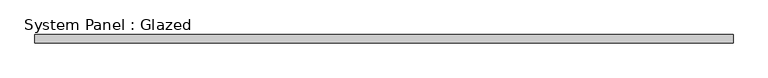
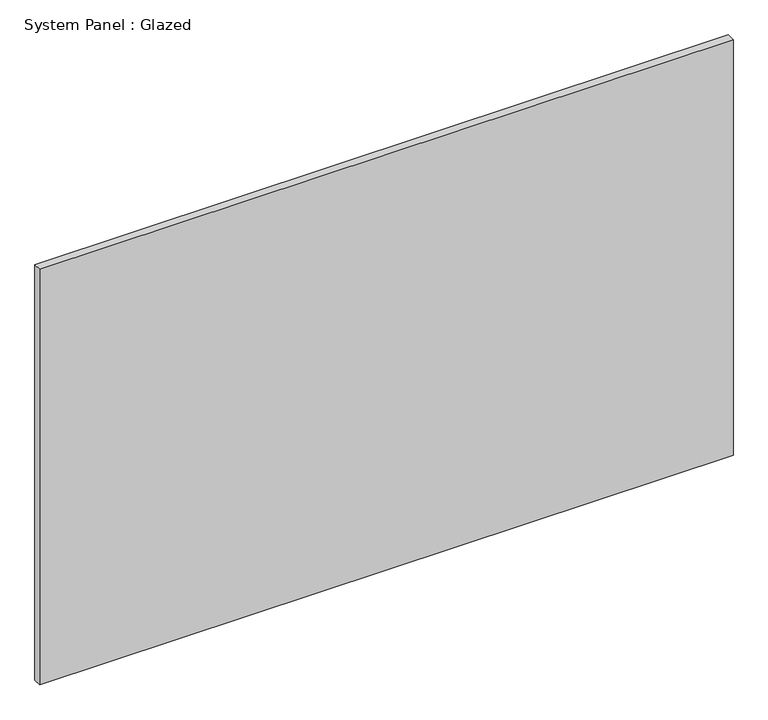
"""IFC4 building model written with IfcOpenShell, lengths in millimetres: plate geometry, System Panel : Glazed."""

from ifc_helpers import new_model, si_unit, origin, origin_with_axes, place, context, project, spatial, polyline, outline, extrude, source, transform, mapped, element, save


def system_panel_glazed_f31d7781(model_context):
    return source(origin(), model_context, "Body", "SweptSolid", [
        extrude(outline(polyline([(1066.8, 19.05), (-1066.8, 19.05), (-1066.8, 44.45), (1066.8, 44.45), (1066.8, 19.05)])), origin_with_axes(), (0.0, 0.0, 1.0), 1351.7614699),
    ])


if __name__ == "__main__":
    model = new_model("IFC4")
    model_context = context("Model", 3, world=origin())
    ifc_project = project(units=[si_unit("LENGTHUNIT", "METRE", prefix="MILLI")], contexts=[model_context])
    site = spatial("IfcSite", under=ifc_project)
    building = spatial("IfcBuilding", under=site)
    placement = place(None, origin())
    system_panel_glazed_shape = system_panel_glazed_f31d7781(model_context)
    element("IfcPlate", 1, ObjectType="System Panel : Glazed", at=placement, inside=building, context=model_context, shape_type="MappedRepresentation", body=[
        mapped(system_panel_glazed_shape, transform((0.0, 0.0, 0.0), x_axis=(1.0, 0.0, 0.0), y_axis=(0.0, 1.0, 0.0), z_axis=(0.0, 0.0, 1.0))),
    ])
    save(model, "model.ifc")

# Revit data of these elements
# Type "System Panel : Glazed"
#   Construction Type Id = "GSP4R"
#   Analytic Construction = "1/8 in Pilkington single glazing"
#   Visual Light Transmittance = 0.9
#   Solar Heat Gain Coefficient = 0.86
#   Heat Transfer Coefficient (U) = 1.18115 BTU/(h·ft²·°F)
#   Define Thermal Properties by = 1
# Element 1 (IfcPlate, "System Panel : Glazed")
#   Materials on its faces: "Glass"
# Materials
#   "Glass": class "Glass", colour RGB 0 128 192, transparency 0.75, Description = "Soda Lime Glass", Cost = 0
